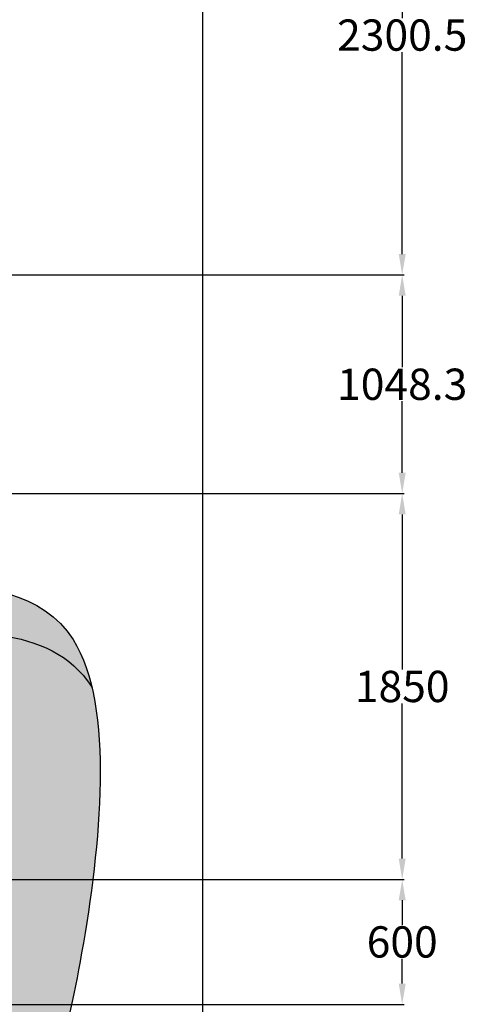
# Model space of a CAD drawing. Units: millimetres. Extents: x 11032 to 26788, y 3406 to 24505.
# Tile 74 of 78: x 24519 to 26666, y 12721 to 17443. Entities that reach past the tile are written whole.
import ezdxf

# ---------------------------------------------------------------- set-up
doc = ezdxf.new("R2010")
doc.units = ezdxf.units.MM
doc.header["$MEASUREMENT"] = 0
doc.layers.add('A-ANNO-DIMS', color=2, linetype='Continuous', lineweight=18)
doc.layers.add('A-ROOF', color=7, linetype='Continuous', lineweight=30)
doc.layers.add('A-ROOF-PATT', color=9, linetype='Continuous', lineweight=13, true_color=0xc7c8ca)
doc.layers.add('A-WALL-CLAD-PATT', color=9, linetype='Continuous', lineweight=13, true_color=0xc7c8ca)
doc.styles.get("Standard").update_dxf_attribs({"font": 'arial.ttf'})
doc.dimstyles.get("Standard").update_dxf_attribs({"dimtxt": 150, "dimasz": 100, "dimexe": 10, "dimexo": 5, "dimgap": 5, "dimtad": 0, "dimtih": 1, "dimtoh": 1, "dimdec": 0, "dimzin": 0, "dimdsep": 46, "dimtxsty": 'Standard', "dimcen": 0.09, "dimadec": 0, "dimazin": 0, "dimtfac": 1, "dimtdec": 0, "dimtofl": 0, "dimtmove": 0, "dimatfit": 3, "dimfxl": 1, "dimtolj": 1, "dimtzin": 0, "dimarcsym": 0})

# ---------------------------------------------------------------- blocks, each defined once
blk = doc.blocks.new('*D36')
at = {"layer": 'A-ANNO-DIMS', "color": 0, "lineweight": -2, "transparency": 16777216}
for p, q in [((12301.3, 17115.9), (12301.3, 24416.9)), ((25397.4, 4466.4), (25397.4, 24416.9)), ((12401.3, 24406.9), (18569.2, 24406.9)), ((25297.4, 24406.9), (19129.5, 24406.9))]:
    blk.add_line(p, q, dxfattribs=at)
at = {"layer": 'A-ANNO-DIMS', "color": 0, "transparency": 16777216}
for points in [[(12401.3, 24423.5), (12401.3, 24390.2), (12301.3, 24406.9)], [(25297.4, 24423.5), (25297.4, 24390.2), (25397.4, 24406.9)]]:
    blk.add_solid(points, dxfattribs=at)
at = {"layer": 'Defpoints', "color": 0, "transparency": 16777216}
for p in [(25397.4, 24406.9), (12301.3, 17110.9), (25397.4, 4461.4)]:
    blk.add_point(p, dxfattribs=at)
at = {"layer": 'A-ANNO-DIMS', "color": 0, "transparency": 16777216, "insert": (18849.3, 24406.9), "char_height": 150, "attachment_point": 5}
blk.add_mtext('\\A1;13096', dxfattribs=at)
blk = doc.blocks.new('*D42')
at = {"layer": 'A-ANNO-DIMS', "color": 0, "lineweight": -2, "transparency": 16777216}
for p, q in [((22752.4, 13320.1), (26363.9, 13320.1)), ((26353.9, 13220.1), (26353.9, 13101.7)), ((26353.9, 12820.1), (26353.9, 12938.5)), ((22752.4, 12720.1), (26363.9, 12720.1))]:
    blk.add_line(p, q, dxfattribs=at)
at = {"layer": 'A-ANNO-DIMS', "color": 0, "transparency": 16777216}
for points in [[(26337.2, 13220.1), (26370.6, 13220.1), (26353.9, 13320.1)], [(26337.2, 12820.1), (26370.6, 12820.1), (26353.9, 12720.1)]]:
    blk.add_solid(points, dxfattribs=at)
at = {"layer": 'Defpoints', "color": 0, "transparency": 16777216}
for p in [(22747.4, 13320.1), (26353.9, 13320.1), (22747.4, 12720.1)]:
    blk.add_point(p, dxfattribs=at)
at = {"layer": 'A-ANNO-DIMS', "color": 0, "transparency": 16777216, "insert": (26353.9, 13020.1), "char_height": 150, "attachment_point": 5}
blk.add_mtext('\\A1;600', dxfattribs=at)
blk = doc.blocks.new('*D43')
at = {"layer": 'A-ANNO-DIMS', "color": 0, "lineweight": -2, "transparency": 16777216}
for p, q in [((22752.4, 15170.1), (26363.9, 15170.1)), ((26353.9, 15070.1), (26353.9, 14326.7)), ((26353.9, 13420.1), (26353.9, 14163.5)), ((22752.4, 13320.1), (26363.9, 13320.1))]:
    blk.add_line(p, q, dxfattribs=at)
at = {"layer": 'A-ANNO-DIMS', "color": 0, "transparency": 16777216}
for points in [[(26337.2, 15070.1), (26370.6, 15070.1), (26353.9, 15170.1)], [(26337.2, 13420.1), (26370.6, 13420.1), (26353.9, 13320.1)]]:
    blk.add_solid(points, dxfattribs=at)
at = {"layer": 'Defpoints', "color": 0, "transparency": 16777216}
for p in [(22747.4, 15170.1), (26353.9, 15170.1), (22747.4, 13320.1)]:
    blk.add_point(p, dxfattribs=at)
at = {"layer": 'A-ANNO-DIMS', "color": 0, "transparency": 16777216, "insert": (26353.9, 14245.1), "char_height": 150, "attachment_point": 5}
blk.add_mtext('\\A1;1850', dxfattribs=at)
blk = doc.blocks.new('*D44')
at = {"layer": 'A-ANNO-DIMS', "color": 0, "lineweight": -2, "transparency": 16777216}
for p, q in [((22902.4, 16218.4), (26363.9, 16218.4)), ((26353.9, 16118.4), (26353.9, 15775.9)), ((26353.9, 15270.1), (26353.9, 15612.6)), ((22752.4, 15170.1), (26363.9, 15170.1))]:
    blk.add_line(p, q, dxfattribs=at)
at = {"layer": 'A-ANNO-DIMS', "color": 0, "transparency": 16777216}
for points in [[(26337.2, 16118.4), (26370.6, 16118.4), (26353.9, 16218.4)], [(26337.2, 15270.1), (26370.6, 15270.1), (26353.9, 15170.1)]]:
    blk.add_solid(points, dxfattribs=at)
at = {"layer": 'Defpoints', "color": 0, "transparency": 16777216}
for p in [(22897.4, 16218.4), (26353.9, 16218.4), (22747.4, 15170.1)]:
    blk.add_point(p, dxfattribs=at)
at = {"layer": 'A-ANNO-DIMS', "color": 0, "transparency": 16777216, "insert": (26353.9, 15694.3), "char_height": 150, "attachment_point": 5}
blk.add_mtext('\\A1;1048.3', dxfattribs=at)
blk = doc.blocks.new('*D45')
at = {"layer": 'A-ANNO-DIMS', "color": 0, "lineweight": -2, "transparency": 16777216}
for p, q in [((13792.4, 18518.9), (26363.9, 18518.9)), ((26353.9, 18418.9), (26353.9, 17450.3)), ((26353.9, 16318.4), (26353.9, 17287)), ((22902.4, 16218.4), (26363.9, 16218.4))]:
    blk.add_line(p, q, dxfattribs=at)
at = {"layer": 'A-ANNO-DIMS', "color": 0, "transparency": 16777216}
for points in [[(26337.2, 18418.9), (26370.6, 18418.9), (26353.9, 18518.9)], [(26337.2, 16318.4), (26370.6, 16318.4), (26353.9, 16218.4)]]:
    blk.add_solid(points, dxfattribs=at)
at = {"layer": 'Defpoints', "color": 0, "transparency": 16777216}
for p in [(13787.4, 18518.9), (26353.9, 18518.9), (22897.4, 16218.4)]:
    blk.add_point(p, dxfattribs=at)
at = {"layer": 'A-ANNO-DIMS', "color": 0, "transparency": 16777216, "insert": (26353.9, 17368.7), "char_height": 150, "attachment_point": 5}
blk.add_mtext('\\A1;2300.5', dxfattribs=at)

msp = doc.modelspace()

# ---------------------------------------------------------------- hatches: boundary and pattern name
at = {"layer": 'A-ROOF-PATT'}
h = msp.add_hatch(color=256, dxfattribs=at)
h.set_gradient(color1=(254, 234, 185), color2=(254, 204, 102), name='HEMISPHERICAL')
edge = h.paths.add_edge_path()
edge.add_spline(control_points=[(22897.404, 11669.966), (22905.925, 11665.421), (23315.936, 11448.075), (24040.798, 11159.928), (24591.756, 12047.169), (24823.737, 12810.982), (24947.403, 13888.961), (24865.187, 14241.353)], knot_values=[3287.74811127, 3287.74811127, 3287.74811127, 3287.74811127, 3313.95061448, 4543.69878516, 5160.49832431, 6201.61230094, 7164.26935092, 7164.26935092, 7164.26935092, 7164.26935092], degree=3, periodic=0)
edge.add_spline(control_points=[(24865.187, 14241.353), (24864.423, 14242.575), (24766.311, 14398.016), (24602.876, 14465.087), (24430.499, 14490.269)], knot_values=[2462.20964139, 2462.20964139, 2462.20964139, 2462.20964139, 2466.8266732, 3052.28296943, 3052.28296943, 3052.28296943, 3052.28296943], degree=3, periodic=0)
edge.add_spline(control_points=[(24430.499, 14490.269), (24425.883, 14491.82), (24421.191, 14493.323), (24402.038, 14499.174), (24386.985, 14503.129), (24351.089, 14511.181), (24329.855, 14514.969), (24285.944, 14521.074), (24263.27, 14523.392), (24216.998, 14526.696), (24193.401, 14527.682), (24156.534, 14528.34), (24143.408, 14528.404), (24117.112, 14528.234), (24103.938, 14528.001), (24070.613, 14527.088), (24050.758, 14526.245), (24021.415, 14524.553), (24011.706, 14523.918), (23966.994, 14520.648), (23932.846, 14517.154), (23866.075, 14508.38), (23833.453, 14503.099), (23769.399, 14490.798), (23737.967, 14483.778), (23675.954, 14468.02), (23645.373, 14459.282), (23584.735, 14440.092), (23554.677, 14429.638), (23494.779, 14407.002), (23464.938, 14394.819), (23420.13, 14375.236), (23405.186, 14368.49), (23382.735, 14358.043), (23375.245, 14354.506), (23363.999, 14349.118), (23360.248, 14347.308), (23354.645, 14344.586), (23352.794, 14343.684), (23350.017, 14342.326), (23349.099, 14341.876), (23346.705, 14340.7), (23345.24, 14339.978), (23338.743, 14336.765), (23333.903, 14334.336), (23322.952, 14328.714), (23316.906, 14325.517), (23304.544, 14318.72), (23298.224, 14315.118), (23284.755, 14307.106), (23277.606, 14302.694), (23262.032, 14292.682), (23253.61, 14287.081), (23235.154, 14274.351), (23225.122, 14267.224), (23200.911, 14249.486), (23186.304, 14238.46), (23150.266, 14210.435), (23128.041, 14192.649), (23080.227, 14153.32), (23055.083, 14132.223), (23027.357, 14108.523)], knot_values=[765.02120011, 765.02120011, 765.02120011, 765.02120011, 788.26421035, 788.26421035, 858.47024111, 858.47024111, 949.55129088, 949.55129088, 1040.63234064, 1040.63234064, 1131.71339041, 1131.71339041, 1181.69353236, 1181.69353236, 1231.67367431, 1231.67367431, 1308.31901537, 1308.31901537, 1346.64168591, 1346.64168591, 1486.09404767, 1486.09404767, 1625.54640943, 1625.54640943, 1764.99877119, 1764.99877119, 1904.45113295, 1904.45113295, 2043.90349471, 2043.90349471, 2183.35585648, 2183.35585648, 2253.08203736, 2253.08203736, 2287.9451278, 2287.9451278, 2305.37667302, 2305.37667302, 2313.97014819, 2313.97014819, 2318.26688578, 2318.26688578, 2325.26983634, 2325.26983634, 2349.68341829, 2349.68341829, 2381.60377634, 2381.60377634, 2413.52413439, 2413.52413439, 2445.44449243, 2445.44449243, 2477.36485048, 2477.36485048, 2509.28520853, 2509.28520853, 2547.80727814, 2547.80727814, 2595.07704725, 2595.07704725, 2638.35089074, 2638.35089074, 2638.35089074, 2638.35089074], degree=3, periodic=0)
edge.add_spline(control_points=[(23027.357, 14108.523), (23027.349, 14108.516), (23027.342, 14108.51), (23027.334, 14108.504), (22984.024, 14071.482), (22940.714, 14034.46), (22897.404, 13997.439)], knot_values=[697.41436256, 697.41436256, 697.41436256, 697.41436256, 697.4261083, 697.4261083, 697.4261083, 765.02120011, 765.02120011, 765.02120011, 765.02120011], degree=3, periodic=0)
edge.add_line((22897.404, 13997.439), (22897.404, 11669.966))
h.paths.add_polyline_path([(23729.349, 12537.488, -1), (23529.349, 12537.488, -1)], flags=16)
h.paths.add_polyline_path([(23963.611, 13699.89, -1), (24163.611, 13699.89, -1)], flags=16)
at = {"layer": 'A-WALL-CLAD-PATT'}
h = msp.add_hatch(color=256, dxfattribs=at)
edge = h.paths.add_edge_path()
edge.add_spline(control_points=[(24865.187, 14241.353), (24844.683, 14329.238), (24708.481, 14689.762), (23980.011, 14777.842), (23439.65, 14624.598), (23111.535, 14443.589), (22897.404, 14260.55)], knot_values=[765.02120011, 765.02120011, 765.02120011, 765.02120011, 1005.10337375, 1880.54593672, 2963.32805357, 3287.74811127, 3287.74811127, 3287.74811127, 3287.74811127], degree=3, periodic=0)
edge.add_line((22897.404, 14260.55), (22897.404, 13997.439))
edge.add_spline(control_points=[(22897.404, 13997.439), (22940.714, 14034.46), (22984.024, 14071.482), (23027.334, 14108.504), (23027.342, 14108.51), (23027.349, 14108.516), (23027.357, 14108.523)], knot_values=[697.41436256, 697.41436256, 697.41436256, 697.41436256, 765.00945437, 765.00945437, 765.00945437, 765.02120011, 765.02120011, 765.02120011, 765.02120011], degree=3, periodic=0)
edge.add_spline(control_points=[(23027.357, 14108.523), (23055.083, 14132.223), (23080.227, 14153.32), (23128.041, 14192.649), (23150.266, 14210.435), (23186.304, 14238.46), (23200.911, 14249.486), (23225.122, 14267.224), (23235.154, 14274.351), (23253.61, 14287.081), (23262.032, 14292.682), (23277.606, 14302.694), (23284.755, 14307.106), (23298.224, 14315.118), (23304.544, 14318.72), (23316.906, 14325.517), (23322.952, 14328.714), (23333.903, 14334.336), (23338.743, 14336.765), (23345.24, 14339.978), (23346.705, 14340.7), (23349.099, 14341.876), (23350.017, 14342.326), (23352.794, 14343.684), (23354.645, 14344.586), (23360.248, 14347.308), (23363.999, 14349.118), (23375.245, 14354.506), (23382.735, 14358.043), (23405.186, 14368.49), (23420.13, 14375.236), (23464.938, 14394.819), (23494.779, 14407.002), (23554.677, 14429.638), (23584.735, 14440.092), (23645.373, 14459.282), (23675.954, 14468.02), (23737.967, 14483.778), (23769.399, 14490.798), (23833.453, 14503.099), (23866.075, 14508.38), (23932.846, 14517.154), (23966.994, 14520.648), (24011.706, 14523.918), (24021.415, 14524.553), (24050.758, 14526.245), (24070.613, 14527.088), (24103.938, 14528.001), (24117.112, 14528.234), (24143.408, 14528.404), (24156.534, 14528.34), (24193.401, 14527.682), (24216.998, 14526.696), (24263.27, 14523.392), (24285.944, 14521.074), (24329.855, 14514.969), (24351.089, 14511.181), (24386.985, 14503.129), (24402.038, 14499.174), (24421.191, 14493.323), (24425.883, 14491.82), (24430.499, 14490.269)], knot_values=[765.02120011, 765.02120011, 765.02120011, 765.02120011, 808.29504361, 808.29504361, 855.56481272, 855.56481272, 894.08688233, 894.08688233, 926.00724037, 926.00724037, 957.92759842, 957.92759842, 989.84795647, 989.84795647, 1021.76831451, 1021.76831451, 1053.68867256, 1053.68867256, 1078.10225451, 1078.10225451, 1085.10520508, 1085.10520508, 1089.40194266, 1089.40194266, 1097.99541784, 1097.99541784, 1115.42696306, 1115.42696306, 1150.2900535, 1150.2900535, 1220.01623438, 1220.01623438, 1359.46859614, 1359.46859614, 1498.9209579, 1498.9209579, 1638.37331966, 1638.37331966, 1777.82568142, 1777.82568142, 1917.27804319, 1917.27804319, 2056.73040495, 2056.73040495, 2095.05307548, 2095.05307548, 2171.69841654, 2171.69841654, 2221.67855849, 2221.67855849, 2271.65870045, 2271.65870045, 2362.73975021, 2362.73975021, 2453.82079998, 2453.82079998, 2544.90184974, 2544.90184974, 2615.10788051, 2615.10788051, 2638.35089074, 2638.35089074, 2638.35089074, 2638.35089074], degree=3, periodic=0)
edge.add_spline(control_points=[(24430.499, 14490.269), (24602.876, 14465.087), (24766.311, 14398.016), (24864.423, 14242.575), (24865.187, 14241.353)], knot_values=[2462.20964139, 2462.20964139, 2462.20964139, 2462.20964139, 3047.66593763, 3052.28296943, 3052.28296943, 3052.28296943, 3052.28296943], degree=3, periodic=0)
h.paths.add_polyline_path([(25397.404, 11120.753), (22897.404, 11120.753), (22897.404, 10520.753), (25197.404, 10520.753), (25197.404, 9359.601), (25397.404, 9359.601)])

# ---------------------------------------------------------------- linework, layer by layer
at = {"layer": 'A-ROOF'}
for points, knots in [([(22897.404, 14260.55), (23111.535, 14443.589), (23439.65, 14624.598), (23980.011, 14777.842), (25027.484, 14651.191), (24844.989, 12880.959), (24591.756, 12047.169), (24040.798, 11159.928), (23315.936, 11448.075), (22905.925, 11665.421), (22897.404, 11669.966)], [765.02120011, 765.02120011, 765.02120011, 765.02120011, 1089.44125781, 2172.22337467, 3047.66593763, 4250.40516126, 5291.51913789, 5908.31867703, 7138.06684772, 7164.26935092, 7164.26935092, 7164.26935092, 7164.26935092]), ([(24430.499, 14490.269), (24602.876, 14465.087), (24766.311, 14398.016), (24864.423, 14242.575), (24865.187, 14241.353)], [2462.20964139, 2462.20964139, 2462.20964139, 2462.20964139, 3047.66593763, 3052.28296943, 3052.28296943, 3052.28296943, 3052.28296943])]:
    msp.add_open_spline(points, degree=3, knots=knots, dxfattribs=at)

# ---------------------------------------------------------------- dimensions: what is measured, and where the dimension line sits
at = {"layer": 'A-ANNO-DIMS'}
dim = msp.add_linear_dim(base=(25397.404, 24406.858), p1=(12301.265, 17110.885), p2=(25397.404, 4461.399), dimstyle='Standard', override={"dimdec": 0, "dimlfac": 1, "dimrnd": 0, "dimzin": 0, "dimdsep": 46, "dimlunit": 2}, dxfattribs=at)
dim.commit()
dim.dimension.update_dxf_attribs({"geometry": '*D36', "text_midpoint": (18849.334, 24406.858)})
for base, p1, p2, override, picture, middle in [((26353.904, 18518.925), (22897.404, 16218.44), (13787.367, 18518.925), {"dimdec": 1, "dimlfac": 1, "dimrnd": 0, "dimzin": 0, "dimdsep": 46, "dimlunit": 2}, '*D45', (26353.904, 17368.682)), ((26353.904, 16218.44), (22747.404, 15170.094), (22897.404, 16218.44), {"dimdec": 1, "dimlfac": 1, "dimrnd": 0, "dimzin": 0, "dimdsep": 46, "dimlunit": 2}, '*D44', (26353.904, 15694.267)), ((26353.904, 15170.094), (22747.404, 13320.07), (22747.404, 15170.094), {"dimdec": 0, "dimlfac": 1, "dimrnd": 0, "dimzin": 0, "dimdsep": 46, "dimlunit": 2}, '*D43', (26353.904, 14245.082)), ((26353.904, 13320.07), (22747.404, 12720.064), (22747.404, 13320.07), {"dimdec": 0, "dimlfac": 1, "dimrnd": 0, "dimzin": 0, "dimdsep": 46, "dimlunit": 2}, '*D42', (26353.904, 13020.067))]:
    dim = msp.add_linear_dim(base=base, p1=p1, p2=p2, angle=90, dimstyle='Standard', override=override, dxfattribs=at)
    dim.commit()
    dim.dimension.update_dxf_attribs({"geometry": picture, "text_midpoint": middle})

doc.saveas('drawing.dxf')
